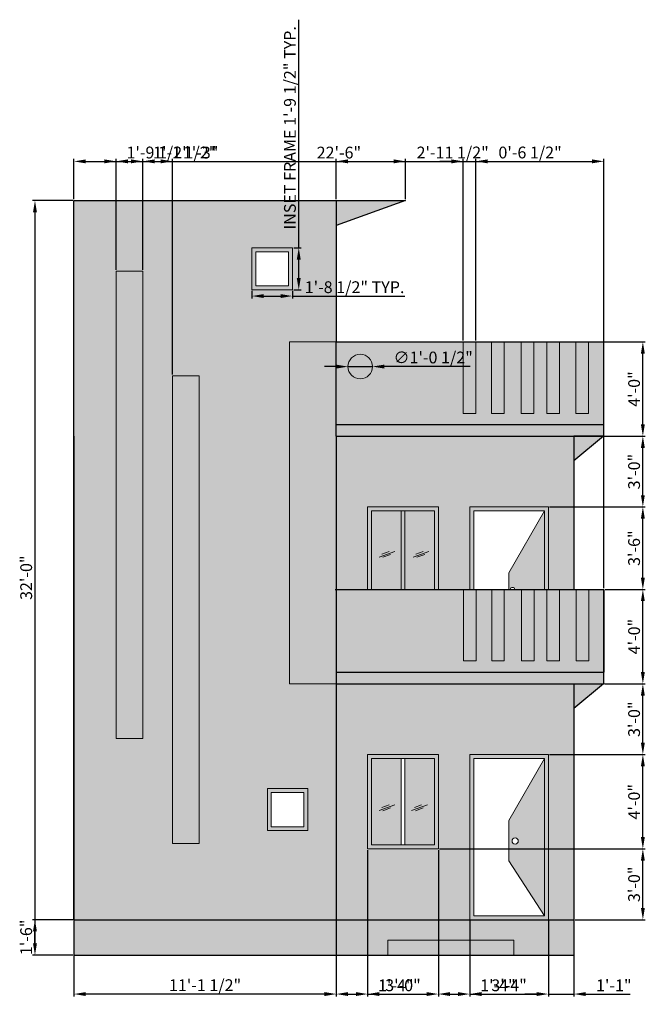
# Model space of a CAD drawing. Units: inches. Extents: x 40559 to 41508, y 131086 to 132358.
# Tile 5 of 5: x 40592 to 40910, y 131857 to 132358. Entities that reach past the tile are written whole.
import ezdxf

# ---------------------------------------------------------------- set-up
doc = ezdxf.new("R2010")
doc.units = ezdxf.units.IN
for name, color, linetype, lineweight in [('A-ANNO-DIMS', 2, 'Continuous', 18), ('A-ELEV', 7, 'Continuous', 30), ('A-ELEV-DETL', 7, 'Continuous', 18), ('A-ELEV-DOOR-PATT', 24, 'Continuous', 13), ('A-ELEV-FRAM-PATT', 7, 'Continuous', 13), ('A-ELEV-OPEN', 7, 'Continuous', 18), ('A-ELEV-RECS-PATT', 250, 'Continuous', 13)]:
    doc.layers.add(name, color=color, linetype=linetype, lineweight=lineweight)
for name, color, linetype, lineweight, true_color in [('A-ELEV-CLAD-PATT', 251, 'Continuous', 13, 0x636466), ('A-ELEV-GLAZ-PATT', 141, 'Continuous', 13, 0xadddf7), ('A-ELEV-TRIM-PATT', 244, 'Continuous', 13, 0x991b1e), ('A-ELEV-WALL-PATT', 254, 'Continuous', 13, 0xfeeab9)]:
    doc.layers.add(name, color=color, linetype=linetype, lineweight=lineweight, true_color=true_color)
doc.styles.get("Standard").update_dxf_attribs({"font": 'arial.ttf'})
doc.dimstyles.new('ISO-25', dxfattribs={"dimtxt": 6, "dimasz": 6, "dimexe": 1.25, "dimexo": 0.625, "dimtad": 1, "dimdec": 0, "dimlunit": 3, "dimtxsty": 'Standard', "dimcen": 2.5, "dimclrd": 1, "dimclre": 1, "dimclrt": 2, "dimadec": 0, "dimazin": 0, "dimtfac": 1, "dimtdec": 0, "dimtmove": 0, "dimatfit": 3, "dimfxl": 1, "dimarcsym": 0})

# ---------------------------------------------------------------- blocks, each defined once
blk = doc.blocks.new('GLAZING-REFLECTION')
for p, q in [((0, 0.1), (8.04, 3.02)), ((1.38, 1.64), (5.11, 3)), ((1.93, 0), (5.91, 1.45))]:
    blk.add_line(p, q)
blk = doc.blocks.new('FACADE-INSET-FRAME')
for points in [[(0, 21.37), (20.63, 21.37), (20.63, 0), (0, 0)], [(2, 19.37), (18.63, 19.37), (18.63, 2), (2, 2)]]:
    blk.add_lwpolyline(points, close=True)
blk = doc.blocks.new('*D62')
at = {"layer": 'A-ANNO-DIMS', "color": 1, "lineweight": -2, "transparency": 16777216}
for p, q in [((40733.88, 132242.44), (40733.88, 132358.49)), ((40731.3, 132242.44), (40735.13, 132242.44)), ((40733.88, 132227.08), (40733.88, 132236.44)), ((40731.3, 132221.08), (40735.13, 132221.08))]:
    blk.add_line(p, q, dxfattribs=at)
at = {"layer": 'A-ANNO-DIMS', "color": 1, "transparency": 16777216}
for points in [[(40732.88, 132236.44), (40734.88, 132236.44), (40733.88, 132242.44)], [(40732.88, 132227.08), (40734.88, 132227.08), (40733.88, 132221.08)]]:
    blk.add_solid(points, dxfattribs=at)
at = {"layer": 'Defpoints', "color": 0, "transparency": 16777216}
for p in [(40730.68, 132242.44), (40733.88, 132242.44), (40730.68, 132221.08)]:
    blk.add_point(p, dxfattribs=at)
at = {"layer": 'A-ANNO-DIMS', "color": 2, "transparency": 16777216, "insert": (40730.16, 132303.47), "char_height": 6, "attachment_point": 5, "rotation": 90}
blk.add_mtext('INSET FRAME 1\'-9 1/2" TYP.', dxfattribs=at)
blk = doc.blocks.new('*D63')
at = {"layer": 'A-ANNO-DIMS', "color": 1, "lineweight": -2, "transparency": 16777216}
for p, q in [((40710.05, 132220.45), (40710.05, 132216.62)), ((40716.05, 132217.87), (40724.68, 132217.87)), ((40730.68, 132220.45), (40730.68, 132216.62)), ((40730.68, 132217.87), (40787.92, 132217.87))]:
    blk.add_line(p, q, dxfattribs=at)
at = {"layer": 'A-ANNO-DIMS', "color": 1, "transparency": 16777216}
for points in [[(40716.05, 132218.87), (40716.05, 132216.87), (40710.05, 132217.87)], [(40724.68, 132218.87), (40724.68, 132216.87), (40730.68, 132217.87)]]:
    blk.add_solid(points, dxfattribs=at)
at = {"layer": 'Defpoints', "color": 0, "transparency": 16777216}
for p in [(40710.05, 132221.08), (40730.68, 132221.08), (40730.68, 132217.87)]:
    blk.add_point(p, dxfattribs=at)
at = {"layer": 'A-ANNO-DIMS', "color": 2, "transparency": 16777216, "insert": (40762.3, 132221.6), "char_height": 6, "attachment_point": 5}
blk.add_mtext('1\'-8 1/2" TYP.', dxfattribs=at)
blk = doc.blocks.new('*D82')
at = {"layer": 'A-ANNO-DIMS', "color": 1, "lineweight": -2, "transparency": 16777216}
for p, q in [((40618.81, 132266.55), (40598.34, 132266.55)), ((40599.59, 132260.55), (40599.59, 131888.55)), ((40618.81, 131882.55), (40598.34, 131882.55))]:
    blk.add_line(p, q, dxfattribs=at)
at = {"layer": 'A-ANNO-DIMS', "color": 1, "transparency": 16777216}
for points in [[(40598.59, 132260.55), (40600.59, 132260.55), (40599.59, 132266.55)], [(40598.59, 131888.55), (40600.59, 131888.55), (40599.59, 131882.55)]]:
    blk.add_solid(points, dxfattribs=at)
at = {"layer": 'Defpoints', "color": 0, "transparency": 16777216}
for p in [(40619.44, 132266.55), (40599.59, 131882.55), (40619.44, 131882.55)]:
    blk.add_point(p, dxfattribs=at)
at = {"layer": 'A-ANNO-DIMS', "color": 2, "transparency": 16777216, "insert": (40595.9, 132074.55), "char_height": 6, "attachment_point": 5, "rotation": 90}
blk.add_mtext('32\'-0"', dxfattribs=at)
blk = doc.blocks.new('*D83')
at = {"layer": 'A-ANNO-DIMS', "color": 1, "lineweight": -2, "transparency": 16777216}
for p, q in [((40619.44, 132267.18), (40619.44, 132287.65)), ((40889.21, 132069.25), (40889.21, 132287.65)), ((40625.44, 132286.4), (40883.21, 132286.4))]:
    blk.add_line(p, q, dxfattribs=at)
at = {"layer": 'A-ANNO-DIMS', "color": 1, "transparency": 16777216}
for points in [[(40625.44, 132287.4), (40625.44, 132285.4), (40619.44, 132286.4)], [(40883.21, 132287.4), (40883.21, 132285.4), (40889.21, 132286.4)]]:
    blk.add_solid(points, dxfattribs=at)
at = {"layer": 'Defpoints', "color": 0, "transparency": 16777216}
for p in [(40889.21, 132286.4), (40619.44, 132266.55), (40889.21, 132068.62)]:
    blk.add_point(p, dxfattribs=at)
at = {"layer": 'A-ANNO-DIMS', "color": 2, "transparency": 16777216, "insert": (40754.32, 132290.09), "char_height": 6, "attachment_point": 5}
blk.add_mtext('22\'-6"', dxfattribs=at)
blk = doc.blocks.new('*D84')
at = {"layer": 'A-ANNO-DIMS', "color": 1, "lineweight": -2, "transparency": 16777216}
for p, q in [((40618.81, 131900.55), (40598.34, 131900.55)), ((40599.59, 131888.55), (40599.59, 131894.55)), ((40618.81, 131882.55), (40598.34, 131882.55))]:
    blk.add_line(p, q, dxfattribs=at)
at = {"layer": 'A-ANNO-DIMS', "color": 1, "transparency": 16777216}
for points in [[(40598.59, 131894.55), (40600.59, 131894.55), (40599.59, 131900.55)], [(40598.59, 131888.55), (40600.59, 131888.55), (40599.59, 131882.55)]]:
    blk.add_solid(points, dxfattribs=at)
at = {"layer": 'Defpoints', "color": 0, "transparency": 16777216}
for p in [(40599.59, 131900.55), (40619.44, 131900.55), (40619.44, 131882.55)]:
    blk.add_point(p, dxfattribs=at)
at = {"layer": 'A-ANNO-DIMS', "color": 2, "transparency": 16777216, "insert": (40595.9, 131891.55), "char_height": 6, "attachment_point": 5, "rotation": 90}
blk.add_mtext('1\'-6"', dxfattribs=at)
blk = doc.blocks.new('*D85')
at = {"layer": 'A-ANNO-DIMS', "color": 1, "lineweight": -2, "transparency": 16777216}
for p, q in [((40889.56, 132020.55), (40910.31, 132020.55)), ((40909.06, 131990.55), (40909.06, 132014.55)), ((40861.56, 131984.55), (40910.31, 131984.55))]:
    blk.add_line(p, q, dxfattribs=at)
at = {"layer": 'A-ANNO-DIMS', "color": 1, "transparency": 16777216}
for points in [[(40908.06, 132014.55), (40910.06, 132014.55), (40909.06, 132020.55)], [(40908.06, 131990.55), (40910.06, 131990.55), (40909.06, 131984.55)]]:
    blk.add_solid(points, dxfattribs=at)
at = {"layer": 'Defpoints', "color": 0, "transparency": 16777216}
for p in [(40888.94, 132020.55), (40909.06, 132020.55), (40860.94, 131984.55)]:
    blk.add_point(p, dxfattribs=at)
at = {"layer": 'A-ANNO-DIMS', "color": 2, "transparency": 16777216, "insert": (40905.37, 132002.55), "char_height": 6, "attachment_point": 5, "rotation": 90}
blk.add_mtext('3\'-0"', dxfattribs=at)
blk = doc.blocks.new('*D86')
at = {"layer": 'A-ANNO-DIMS', "color": 1, "lineweight": -2, "transparency": 16777216}
for p, q in [((40889.83, 132068.62), (40910.31, 132068.62)), ((40909.06, 132026.55), (40909.06, 132062.62)), ((40889.56, 132020.55), (40910.31, 132020.55))]:
    blk.add_line(p, q, dxfattribs=at)
at = {"layer": 'A-ANNO-DIMS', "color": 1, "transparency": 16777216}
for points in [[(40908.06, 132062.62), (40910.06, 132062.62), (40909.06, 132068.62)], [(40908.06, 132026.55), (40910.06, 132026.55), (40909.06, 132020.55)]]:
    blk.add_solid(points, dxfattribs=at)
at = {"layer": 'Defpoints', "color": 0, "transparency": 16777216}
for p in [(40889.21, 132068.62), (40909.06, 132068.62), (40888.94, 132020.55)]:
    blk.add_point(p, dxfattribs=at)
at = {"layer": 'A-ANNO-DIMS', "color": 2, "transparency": 16777216, "insert": (40905.37, 132044.59), "char_height": 6, "attachment_point": 5, "rotation": 90}
blk.add_mtext('4\'-0"', dxfattribs=at)
blk = doc.blocks.new('*D87')
at = {"layer": 'A-ANNO-DIMS', "color": 1, "lineweight": -2, "transparency": 16777216}
for p, q in [((40861.56, 132110.55), (40910.31, 132110.55)), ((40909.06, 132074.62), (40909.06, 132104.55)), ((40889.83, 132068.62), (40910.31, 132068.62))]:
    blk.add_line(p, q, dxfattribs=at)
at = {"layer": 'A-ANNO-DIMS', "color": 1, "transparency": 16777216}
for points in [[(40908.06, 132104.55), (40910.06, 132104.55), (40909.06, 132110.55)], [(40908.06, 132074.62), (40910.06, 132074.62), (40909.06, 132068.62)]]:
    blk.add_solid(points, dxfattribs=at)
at = {"layer": 'Defpoints', "color": 0, "transparency": 16777216}
for p in [(40860.94, 132110.55), (40909.06, 132110.55), (40889.21, 132068.62)]:
    blk.add_point(p, dxfattribs=at)
at = {"layer": 'A-ANNO-DIMS', "color": 2, "transparency": 16777216, "insert": (40905.37, 132089.59), "char_height": 6, "attachment_point": 5, "rotation": 90}
blk.add_mtext('3\'-6"', dxfattribs=at)
blk = doc.blocks.new('*D88')
at = {"layer": 'A-ANNO-DIMS', "color": 1, "lineweight": -2, "transparency": 16777216}
for p, q in [((40889.56, 132146.55), (40910.31, 132146.55)), ((40909.06, 132116.55), (40909.06, 132140.55)), ((40861.56, 132110.55), (40910.31, 132110.55))]:
    blk.add_line(p, q, dxfattribs=at)
at = {"layer": 'A-ANNO-DIMS', "color": 1, "transparency": 16777216}
for points in [[(40908.06, 132140.55), (40910.06, 132140.55), (40909.06, 132146.55)], [(40908.06, 132116.55), (40910.06, 132116.55), (40909.06, 132110.55)]]:
    blk.add_solid(points, dxfattribs=at)
at = {"layer": 'Defpoints', "color": 0, "transparency": 16777216}
for p in [(40888.94, 132146.55), (40909.06, 132146.55), (40860.94, 132110.55)]:
    blk.add_point(p, dxfattribs=at)
at = {"layer": 'A-ANNO-DIMS', "color": 2, "transparency": 16777216, "insert": (40905.37, 132128.55), "char_height": 6, "attachment_point": 5, "rotation": 90}
blk.add_mtext('3\'-0"', dxfattribs=at)
blk = doc.blocks.new('*D89')
at = {"layer": 'A-ANNO-DIMS', "color": 1, "lineweight": -2, "transparency": 16777216}
for p, q in [((40889.56, 132194.55), (40910.31, 132194.55)), ((40909.06, 132152.55), (40909.06, 132188.55)), ((40889.56, 132146.55), (40910.31, 132146.55))]:
    blk.add_line(p, q, dxfattribs=at)
at = {"layer": 'A-ANNO-DIMS', "color": 1, "transparency": 16777216}
for points in [[(40908.06, 132188.55), (40910.06, 132188.55), (40909.06, 132194.55)], [(40908.06, 132152.55), (40910.06, 132152.55), (40909.06, 132146.55)]]:
    blk.add_solid(points, dxfattribs=at)
at = {"layer": 'Defpoints', "color": 0, "transparency": 16777216}
for p in [(40888.94, 132194.55), (40909.06, 132194.55), (40888.94, 132146.55)]:
    blk.add_point(p, dxfattribs=at)
at = {"layer": 'A-ANNO-DIMS', "color": 2, "transparency": 16777216, "insert": (40905.37, 132170.55), "char_height": 6, "attachment_point": 5, "rotation": 90}
blk.add_mtext('4\'-0"', dxfattribs=at)
blk = doc.blocks.new('*D90')
at = {"layer": 'A-ANNO-DIMS', "color": 1, "lineweight": -2, "transparency": 16777216}
for p, q in [((40619.44, 131899.93), (40619.44, 131861.45)), ((40752.94, 131899.93), (40752.94, 131861.45)), ((40746.94, 131862.7), (40625.44, 131862.7))]:
    blk.add_line(p, q, dxfattribs=at)
at = {"layer": 'A-ANNO-DIMS', "color": 1, "transparency": 16777216}
for points in [[(40625.44, 131863.7), (40625.44, 131861.7), (40619.44, 131862.7)], [(40746.94, 131863.7), (40746.94, 131861.7), (40752.94, 131862.7)]]:
    blk.add_solid(points, dxfattribs=at)
at = {"layer": 'Defpoints', "color": 0, "transparency": 16777216}
for p in [(40619.44, 131900.55), (40752.94, 131900.55), (40619.44, 131862.7)]:
    blk.add_point(p, dxfattribs=at)
at = {"layer": 'A-ANNO-DIMS', "color": 2, "transparency": 16777216, "insert": (40686.19, 131866.43), "char_height": 6, "attachment_point": 5}
blk.add_mtext('11\'-1 1/2"', dxfattribs=at)
blk = doc.blocks.new('*D91')
at = {"layer": 'A-ANNO-DIMS', "color": 1, "lineweight": -2, "transparency": 16777216}
for p, q in [((40768.94, 131935.93), (40768.94, 131861.45)), ((40752.94, 131899.93), (40752.94, 131861.45)), ((40758.94, 131862.7), (40762.94, 131862.7)), ((40768.94, 131862.7), (40791.57, 131862.7))]:
    blk.add_line(p, q, dxfattribs=at)
at = {"layer": 'A-ANNO-DIMS', "color": 1, "transparency": 16777216}
for points in [[(40758.94, 131863.7), (40758.94, 131861.7), (40752.94, 131862.7)], [(40762.94, 131863.7), (40762.94, 131861.7), (40768.94, 131862.7)]]:
    blk.add_solid(points, dxfattribs=at)
at = {"layer": 'Defpoints', "color": 0, "transparency": 16777216}
for p in [(40768.94, 131936.55), (40752.94, 131900.55), (40768.94, 131862.7)]:
    blk.add_point(p, dxfattribs=at)
at = {"layer": 'A-ANNO-DIMS', "color": 2, "transparency": 16777216, "insert": (40783.26, 131866.34), "char_height": 6, "attachment_point": 5}
blk.add_mtext('1\'-4"', dxfattribs=at)
blk = doc.blocks.new('*D92')
at = {"layer": 'A-ANNO-DIMS', "color": 1, "lineweight": -2, "transparency": 16777216}
for p, q in [((40768.94, 131935.93), (40768.94, 131861.45)), ((40804.94, 131935.93), (40804.94, 131861.45)), ((40774.94, 131862.7), (40798.94, 131862.7))]:
    blk.add_line(p, q, dxfattribs=at)
at = {"layer": 'A-ANNO-DIMS', "color": 1, "transparency": 16777216}
for points in [[(40774.94, 131863.7), (40774.94, 131861.7), (40768.94, 131862.7)], [(40798.94, 131863.7), (40798.94, 131861.7), (40804.94, 131862.7)]]:
    blk.add_solid(points, dxfattribs=at)
at = {"layer": 'Defpoints', "color": 0, "transparency": 16777216}
for p in [(40768.94, 131936.55), (40804.94, 131936.55), (40804.94, 131862.7)]:
    blk.add_point(p, dxfattribs=at)
at = {"layer": 'A-ANNO-DIMS', "color": 2, "transparency": 16777216, "insert": (40786.94, 131866.39), "char_height": 6, "attachment_point": 5}
blk.add_mtext('3\'-0"', dxfattribs=at)
blk = doc.blocks.new('*D93')
at = {"layer": 'A-ANNO-DIMS', "color": 1, "lineweight": -2, "transparency": 16777216}
for p, q in [((40804.94, 131935.93), (40804.94, 131861.45)), ((40820.94, 131899.93), (40820.94, 131861.45)), ((40810.94, 131862.7), (40814.94, 131862.7)), ((40820.94, 131862.7), (40843.57, 131862.7))]:
    blk.add_line(p, q, dxfattribs=at)
at = {"layer": 'A-ANNO-DIMS', "color": 1, "transparency": 16777216}
for points in [[(40810.94, 131863.7), (40810.94, 131861.7), (40804.94, 131862.7)], [(40814.94, 131863.7), (40814.94, 131861.7), (40820.94, 131862.7)]]:
    blk.add_solid(points, dxfattribs=at)
at = {"layer": 'Defpoints', "color": 0, "transparency": 16777216}
for p in [(40804.94, 131936.55), (40820.94, 131900.55), (40820.94, 131862.7)]:
    blk.add_point(p, dxfattribs=at)
at = {"layer": 'A-ANNO-DIMS', "color": 2, "transparency": 16777216, "insert": (40835.26, 131866.34), "char_height": 6, "attachment_point": 5}
blk.add_mtext('1\'-4"', dxfattribs=at)
blk = doc.blocks.new('*D94')
at = {"layer": 'A-ANNO-DIMS', "color": 1, "lineweight": -2, "transparency": 16777216}
for p, q in [((40820.94, 131899.93), (40820.94, 131861.45)), ((40860.94, 131899.93), (40860.94, 131861.45)), ((40826.94, 131862.7), (40854.94, 131862.7))]:
    blk.add_line(p, q, dxfattribs=at)
at = {"layer": 'A-ANNO-DIMS', "color": 1, "transparency": 16777216}
for points in [[(40826.94, 131863.7), (40826.94, 131861.7), (40820.94, 131862.7)], [(40854.94, 131863.7), (40854.94, 131861.7), (40860.94, 131862.7)]]:
    blk.add_solid(points, dxfattribs=at)
at = {"layer": 'Defpoints', "color": 0, "transparency": 16777216}
for p in [(40820.94, 131900.55), (40860.94, 131900.55), (40860.94, 131862.7)]:
    blk.add_point(p, dxfattribs=at)
at = {"layer": 'A-ANNO-DIMS', "color": 2, "transparency": 16777216, "insert": (40840.94, 131866.39), "char_height": 6, "attachment_point": 5}
blk.add_mtext('3\'-4"', dxfattribs=at)
blk = doc.blocks.new('*D95')
at = {"layer": 'A-ANNO-DIMS', "color": 1, "lineweight": -2, "transparency": 16777216}
for p, q in [((40860.94, 131899.93), (40860.94, 131861.45)), ((40873.94, 131899.93), (40873.94, 131861.45)), ((40854.94, 131862.7), (40848.94, 131862.7)), ((40860.94, 131862.7), (40873.94, 131862.7)), ((40879.94, 131862.7), (40902.57, 131862.7))]:
    blk.add_line(p, q, dxfattribs=at)
at = {"layer": 'A-ANNO-DIMS', "color": 1, "transparency": 16777216}
for points in [[(40854.94, 131863.7), (40854.94, 131861.7), (40860.94, 131862.7)], [(40879.94, 131863.7), (40879.94, 131861.7), (40873.94, 131862.7)]]:
    blk.add_solid(points, dxfattribs=at)
at = {"layer": 'Defpoints', "color": 0, "transparency": 16777216}
for p in [(40860.94, 131900.55), (40873.94, 131900.55), (40873.94, 131862.7)]:
    blk.add_point(p, dxfattribs=at)
at = {"layer": 'A-ANNO-DIMS', "color": 2, "transparency": 16777216, "insert": (40894.26, 131866.34), "char_height": 6, "attachment_point": 5}
blk.add_mtext('1\'-1"', dxfattribs=at)
blk = doc.blocks.new('*D96')
at = {"layer": 'A-ANNO-DIMS', "color": 1, "lineweight": -2, "transparency": 16777216}
for p, q in [((40805.56, 131936.55), (40910.31, 131936.55)), ((40909.06, 131906.55), (40909.06, 131930.55)), ((40874.56, 131900.55), (40910.31, 131900.55))]:
    blk.add_line(p, q, dxfattribs=at)
at = {"layer": 'A-ANNO-DIMS', "color": 1, "transparency": 16777216}
for points in [[(40908.06, 131930.55), (40910.06, 131930.55), (40909.06, 131936.55)], [(40908.06, 131906.55), (40910.06, 131906.55), (40909.06, 131900.55)]]:
    blk.add_solid(points, dxfattribs=at)
at = {"layer": 'Defpoints', "color": 0, "transparency": 16777216}
for p in [(40804.94, 131936.55), (40909.06, 131936.55), (40873.94, 131900.55)]:
    blk.add_point(p, dxfattribs=at)
at = {"layer": 'A-ANNO-DIMS', "color": 2, "transparency": 16777216, "insert": (40905.37, 131918.55), "char_height": 6, "attachment_point": 5, "rotation": 90}
blk.add_mtext('3\'-0"', dxfattribs=at)
blk = doc.blocks.new('*D97')
at = {"layer": 'A-ANNO-DIMS', "color": 1, "lineweight": -2, "transparency": 16777216}
for p, q in [((40861.56, 131984.55), (40910.31, 131984.55)), ((40909.06, 131942.55), (40909.06, 131978.55)), ((40805.56, 131936.55), (40910.31, 131936.55))]:
    blk.add_line(p, q, dxfattribs=at)
at = {"layer": 'A-ANNO-DIMS', "color": 1, "transparency": 16777216}
for points in [[(40908.06, 131978.55), (40910.06, 131978.55), (40909.06, 131984.55)], [(40908.06, 131942.55), (40910.06, 131942.55), (40909.06, 131936.55)]]:
    blk.add_solid(points, dxfattribs=at)
at = {"layer": 'Defpoints', "color": 0, "transparency": 16777216}
for p in [(40860.94, 131984.55), (40909.06, 131984.55), (40804.94, 131936.55)]:
    blk.add_point(p, dxfattribs=at)
at = {"layer": 'A-ANNO-DIMS', "color": 2, "transparency": 16777216, "insert": (40905.37, 131960.55), "char_height": 6, "attachment_point": 5, "rotation": 90}
blk.add_mtext('4\'-0"', dxfattribs=at)
blk = doc.blocks.new('*D98')
at = {"layer": 'A-ANNO-DIMS', "color": 1, "lineweight": -2, "transparency": 16777216}
for p, q in [((40817.63, 132195.18), (40817.63, 132287.65)), ((40824.05, 132195.18), (40824.05, 132287.65)), ((40811.63, 132286.4), (40805.63, 132286.4)), ((40817.63, 132286.4), (40824.05, 132286.4)), ((40830.05, 132286.4), (40867.23, 132286.4))]:
    blk.add_line(p, q, dxfattribs=at)
at = {"layer": 'A-ANNO-DIMS', "color": 1, "transparency": 16777216}
for points in [[(40811.63, 132287.4), (40811.63, 132285.4), (40817.63, 132286.4)], [(40830.05, 132287.4), (40830.05, 132285.4), (40824.05, 132286.4)]]:
    blk.add_solid(points, dxfattribs=at)
at = {"layer": 'Defpoints', "color": 0, "transparency": 16777216}
for p in [(40824.05, 132286.4), (40817.63, 132194.55), (40824.05, 132194.55)]:
    blk.add_point(p, dxfattribs=at)
at = {"layer": 'A-ANNO-DIMS', "color": 2, "transparency": 16777216, "insert": (40851.64, 132290.13), "char_height": 6, "attachment_point": 5}
blk.add_mtext('0\'-6 1/2"', dxfattribs=at)
blk = doc.blocks.new('*D99')
at = {"layer": 'A-ANNO-DIMS', "color": 1, "lineweight": -2, "transparency": 16777216}
for p, q in [((40752.94, 132267.18), (40752.94, 132287.65)), ((40788.26, 132267.18), (40788.26, 132287.65)), ((40758.94, 132286.4), (40782.26, 132286.4)), ((40788.26, 132286.4), (40830.21, 132286.4))]:
    blk.add_line(p, q, dxfattribs=at)
at = {"layer": 'A-ANNO-DIMS', "color": 1, "transparency": 16777216}
for points in [[(40758.94, 132287.4), (40758.94, 132285.4), (40752.94, 132286.4)], [(40782.26, 132287.4), (40782.26, 132285.4), (40788.26, 132286.4)]]:
    blk.add_solid(points, dxfattribs=at)
at = {"layer": 'Defpoints', "color": 0, "transparency": 16777216}
for p in [(40788.26, 132286.4), (40752.94, 132266.55), (40788.26, 132266.55)]:
    blk.add_point(p, dxfattribs=at)
at = {"layer": 'A-ANNO-DIMS', "color": 2, "transparency": 16777216, "insert": (40812.23, 132290.13), "char_height": 6, "attachment_point": 5}
blk.add_mtext('2\'-11 1/2"', dxfattribs=at)
blk = doc.blocks.new('*D100')
at = {"layer": 'A-ANNO-DIMS', "color": 1, "lineweight": -2, "transparency": 16777216}
for p, q in [((40640.97, 132231.22), (40640.97, 132287.65)), ((40654.52, 132231.22), (40654.52, 132287.65)), ((40646.97, 132286.4), (40648.52, 132286.4)), ((40654.52, 132286.4), (40691.13, 132286.4))]:
    blk.add_line(p, q, dxfattribs=at)
at = {"layer": 'A-ANNO-DIMS', "color": 1, "transparency": 16777216}
for points in [[(40646.97, 132287.4), (40646.97, 132285.4), (40640.97, 132286.4)], [(40648.52, 132287.4), (40648.52, 132285.4), (40654.52, 132286.4)]]:
    blk.add_solid(points, dxfattribs=at)
at = {"layer": 'Defpoints', "color": 0, "transparency": 16777216}
for p in [(40654.52, 132286.4), (40640.97, 132230.6), (40654.52, 132230.6)]:
    blk.add_point(p, dxfattribs=at)
at = {"layer": 'A-ANNO-DIMS', "color": 2, "transparency": 16777216, "insert": (40675.82, 132290.13), "char_height": 6, "attachment_point": 5}
blk.add_mtext('1\'-1 1/2"', dxfattribs=at)
blk = doc.blocks.new('*D101')
at = {"layer": 'A-ANNO-DIMS', "color": 1, "lineweight": -2, "transparency": 16777216}
for p, q in [((40619.44, 132267.18), (40619.44, 132287.65)), ((40640.97, 132231.22), (40640.97, 132287.65)), ((40625.44, 132286.4), (40634.97, 132286.4)), ((40640.97, 132286.4), (40677.58, 132286.4))]:
    blk.add_line(p, q, dxfattribs=at)
at = {"layer": 'A-ANNO-DIMS', "color": 1, "transparency": 16777216}
for points in [[(40625.44, 132287.4), (40625.44, 132285.4), (40619.44, 132286.4)], [(40634.97, 132287.4), (40634.97, 132285.4), (40640.97, 132286.4)]]:
    blk.add_solid(points, dxfattribs=at)
at = {"layer": 'Defpoints', "color": 0, "transparency": 16777216}
for p in [(40640.97, 132286.4), (40619.44, 132266.55), (40640.97, 132230.6)]:
    blk.add_point(p, dxfattribs=at)
at = {"layer": 'A-ANNO-DIMS', "color": 2, "transparency": 16777216, "insert": (40662.28, 132290.13), "char_height": 6, "attachment_point": 5}
blk.add_mtext('1\'-9 1/2"', dxfattribs=at)
blk = doc.blocks.new('*D102')
at = {"layer": 'A-ANNO-DIMS', "color": 1, "lineweight": -2, "transparency": 16777216}
for p, q in [((40654.52, 132231.22), (40654.52, 132287.65)), ((40669.6, 132177.9), (40669.6, 132287.65)), ((40660.52, 132286.4), (40663.6, 132286.4)), ((40669.6, 132286.4), (40692.23, 132286.4))]:
    blk.add_line(p, q, dxfattribs=at)
at = {"layer": 'A-ANNO-DIMS', "color": 1, "transparency": 16777216}
for points in [[(40660.52, 132287.4), (40660.52, 132285.4), (40654.52, 132286.4)], [(40663.6, 132287.4), (40663.6, 132285.4), (40669.6, 132286.4)]]:
    blk.add_solid(points, dxfattribs=at)
at = {"layer": 'Defpoints', "color": 0, "transparency": 16777216}
for p in [(40669.6, 132286.4), (40654.52, 132230.6), (40669.6, 132177.27)]:
    blk.add_point(p, dxfattribs=at)
at = {"layer": 'A-ANNO-DIMS', "color": 2, "transparency": 16777216, "insert": (40683.92, 132290.09), "char_height": 6, "attachment_point": 5}
blk.add_mtext('1\'-3"', dxfattribs=at)
blk = doc.blocks.new('*D106')
at = {"layer": 'A-ANNO-DIMS', "color": 1, "lineweight": -2, "transparency": 16777216}
for p, q in [((40752.93, 132181.97), (40746.93, 132181.97)), ((40758.93, 132181.97), (40771.44, 132181.97)), ((40821.15, 132181.97), (40777.44, 132181.97))]:
    blk.add_line(p, q, dxfattribs=at)
at = {"layer": 'A-ANNO-DIMS', "color": 1, "transparency": 16777216}
for points in [[(40752.93, 132182.97), (40752.93, 132180.97), (40758.93, 132181.97)], [(40777.44, 132182.97), (40777.44, 132180.97), (40771.44, 132181.97)]]:
    blk.add_solid(points, dxfattribs=at)
at = {"layer": 'Defpoints', "color": 0, "transparency": 16777216}
for p in [(40758.93, 132181.97), (40771.44, 132181.97)]:
    blk.add_point(p, dxfattribs=at)
at = {"layer": 'A-ANNO-DIMS', "color": 2, "transparency": 16777216, "insert": (40802.3, 132185.83), "char_height": 6, "attachment_point": 5, "rotation": 0.001}
blk.add_mtext('∅1\'-0 1/2"', dxfattribs=at)

msp = doc.modelspace()

# ---------------------------------------------------------------- hatches: boundary and pattern name
at = {"layer": 'A-ELEV-CLAD-PATT'}
h = msp.add_hatch(color=256, dxfattribs=at)
h.dxf.hatch_style = 1
h.paths.add_polyline_path([(40729.2, 132194.55), (40752.94, 132194.55), (40752.94, 132266.55), (40619.44, 132266.55), (40619.44, 132194.55), (40619.44, 132146.55), (40619.44, 132020.55), (40619.44, 131900.55), (40752.94, 131900.55), (40752.94, 132020.55), (40729.2, 132020.55)])
h.paths.add_polyline_path([(40683.15, 132177.27), (40683.15, 131939.36), (40669.6, 131939.36), (40669.6, 132177.27)], flags=16)
h.paths.add_polyline_path([(40710.05, 132221.08), (40710.05, 132242.44), (40730.68, 132242.44), (40730.68, 132221.08)], flags=16)
h.paths.add_polyline_path([(40712.05, 132223.08), (40712.05, 132240.44), (40728.68, 132240.44), (40728.68, 132223.08)], flags=0)
h.paths.add_polyline_path([(40654.52, 131992.69), (40640.97, 131992.69), (40640.97, 132230.6), (40654.52, 132230.6)], flags=16)
h.paths.add_polyline_path([(40717.89, 131967.22), (40738.52, 131967.22), (40738.52, 131945.85), (40717.89, 131945.85)], flags=16)
h.paths.add_polyline_path([(40719.89, 131965.22), (40736.52, 131965.22), (40736.52, 131947.85), (40719.89, 131947.85)], flags=0)
h = msp.add_hatch(color=256, dxfattribs=at)
h.dxf.hatch_style = 1
h.paths.add_polyline_path([(40817.69, 132068.55), (40752.94, 132068.55), (40752.94, 132026.55), (40888.94, 132026.55), (40888.94, 132068.55), (40881.5, 132068.55), (40881.5, 132032.18), (40875.08, 132032.18), (40875.08, 132068.55), (40873.94, 132068.55), (40866.62, 132068.55), (40866.62, 132032.18), (40860.2, 132032.18), (40860.2, 132068.55), (40853.65, 132068.55), (40853.65, 132032.18), (40847.23, 132032.18), (40847.23, 132068.55), (40838.53, 132068.55), (40838.53, 132032.18), (40832.1, 132032.18), (40832.1, 132068.55), (40824.12, 132068.55), (40824.12, 132032.18), (40817.69, 132032.18)])
h.paths.add_polyline_path([(40817.63, 132194.55), (40752.94, 132194.55), (40752.94, 132152.55), (40888.94, 132152.55), (40888.94, 132194.55), (40881.44, 132194.55), (40881.44, 132158.11), (40875.01, 132158.11), (40875.01, 132194.55), (40866.56, 132194.55), (40866.56, 132158.11), (40860.13, 132158.11), (40860.13, 132194.55), (40853.59, 132194.55), (40853.59, 132158.11), (40847.16, 132158.11), (40847.16, 132194.55), (40838.46, 132194.55), (40838.46, 132158.11), (40832.03, 132158.11), (40832.03, 132194.55), (40824.05, 132194.55), (40824.05, 132158.11), (40817.63, 132158.11)])
h.paths.add_polyline_path([(40758.93, 132181.97, -1), (40771.44, 132181.97, -1)], flags=16)
h = msp.add_hatch(color=256, dxfattribs=at)
h.dxf.hatch_style = 1
h.paths.add_polyline_path([(40873.94, 131900.55), (40619.44, 131900.55), (40619.44, 131882.55), (40779.29, 131882.55), (40779.29, 131890.06), (40843.37, 131890.06), (40843.37, 131882.55), (40873.94, 131882.55)])
at = {"layer": 'A-ELEV-DOOR-PATT'}
h = msp.add_hatch(color=256, dxfattribs=at)
h.dxf.hatch_style = 1
h.paths.add_polyline_path([(40858.94, 131982.55), (40840.76, 131951.07), (40840.76, 131930.45), (40858.94, 131902.55)])
h.paths.add_polyline_path([(40845.62, 131940.52, -1), (40842.44, 131940.52, -1)], flags=16)
h.paths.add_polyline_path([(40858.94, 132108.55), (40840.76, 132077.07), (40840.76, 132068.55), (40841.6, 132068.55, -1), (40843.79, 132068.55), (40858.94, 132068.55)])
at = {"layer": 'A-ELEV-FRAM-PATT'}
h = msp.add_hatch(color=256, dxfattribs=at)
h.dxf.hatch_style = 1
h.paths.add_polyline_path([(40804.94, 132110.55), (40768.94, 132110.55), (40768.94, 132068.55), (40770.94, 132068.55), (40770.94, 132108.55), (40802.94, 132108.55), (40802.94, 132068.55), (40804.94, 132068.55)])
h.paths.add_polyline_path([(40787.94, 132108.55), (40785.94, 132108.55), (40785.94, 132068.55), (40787.94, 132068.55)], flags=17)
h.paths.add_polyline_path([(40804.94, 131984.55), (40768.94, 131984.55), (40768.94, 131936.55), (40804.94, 131936.55)])
h.paths.add_polyline_path([(40802.94, 131982.55), (40802.94, 131938.55), (40770.94, 131938.55), (40770.94, 131982.55)], flags=16)
h.paths.add_polyline_path([(40787.94, 131982.55), (40785.94, 131982.55), (40785.94, 131938.55), (40787.94, 131938.55)], flags=0)
h = msp.add_hatch(color=256, dxfattribs=at)
h.dxf.hatch_style = 1
h.paths.add_polyline_path([(40860.94, 132110.55), (40820.94, 132110.55), (40820.94, 132068.55), (40822.94, 132068.55), (40822.94, 132108.55), (40858.94, 132108.55), (40858.94, 132068.55), (40860.94, 132068.55)])
h.paths.add_polyline_path([(40860.94, 131984.55), (40820.94, 131984.55), (40820.94, 131900.55), (40860.94, 131900.55)])
h.paths.add_polyline_path([(40858.94, 131982.55), (40858.94, 131902.55), (40822.94, 131902.55), (40822.94, 131982.55)], flags=16)
h.paths.add_polyline_path([(40845.62, 131940.52, -1), (40842.44, 131940.52, -1)], flags=0)
at = {"layer": 'A-ELEV-GLAZ-PATT'}
h = msp.add_hatch(color=256, dxfattribs=at)
h.dxf.hatch_style = 1
h.paths.add_polyline_path([(40785.94, 132108.55), (40770.94, 132108.55), (40770.94, 132068.55), (40785.94, 132068.55)])
h.paths.add_polyline_path([(40802.94, 132108.55), (40787.94, 132108.55), (40787.94, 132068.55), (40802.94, 132068.55)])
h.paths.add_polyline_path([(40785.94, 131982.55), (40770.94, 131982.55), (40770.94, 131938.55), (40785.94, 131938.55)])
h.paths.add_polyline_path([(40802.94, 131982.55), (40787.94, 131982.55), (40787.94, 131938.55), (40802.94, 131938.55)])
at = {"layer": 'A-ELEV-RECS-PATT'}
h = msp.add_hatch(color=256, dxfattribs=at)
h.dxf.hatch_style = 1
h.paths.add_polyline_path([(40788.26, 132266.55), (40777.38, 132266.55), (40752.94, 132266.55), (40752.94, 132253.7)])
h = msp.add_hatch(color=256, dxfattribs=at)
h.dxf.hatch_style = 1
h.paths.add_polyline_path([(40654.52, 132230.6), (40640.97, 132230.6), (40640.97, 131992.69), (40654.52, 131992.69)])
h = msp.add_hatch(color=256, dxfattribs=at)
h.dxf.hatch_style = 1
h.paths.add_polyline_path([(40683.15, 132177.27), (40669.6, 132177.27), (40669.6, 131939.36), (40683.15, 131939.36)])
h = msp.add_hatch(color=256, dxfattribs=at)
h.dxf.hatch_style = 1
h.paths.add_polyline_path([(40888.94, 132146.55), (40873.94, 132146.55), (40873.94, 132133.97)])
h.paths.add_polyline_path([(40888.94, 132020.55), (40873.94, 132020.55), (40873.94, 132007.97)])
h = msp.add_hatch(color=256, dxfattribs=at)
h.dxf.hatch_style = 1
h.paths.add_polyline_path([(40843.37, 131890.06), (40779.29, 131890.06), (40779.29, 131882.55), (40843.37, 131882.55)])
at = {"layer": 'A-ELEV-TRIM-PATT'}
h = msp.add_hatch(color=256, dxfattribs=at)
h.dxf.hatch_style = 1
h.paths.add_polyline_path([(40738.52, 131967.22), (40717.89, 131967.22), (40717.89, 131945.85), (40738.52, 131945.85)])
h.paths.add_polyline_path([(40736.52, 131965.22), (40736.52, 131947.85), (40719.89, 131947.85), (40719.89, 131965.22)], flags=16)
h.paths.add_polyline_path([(40730.68, 132242.44), (40710.05, 132242.44), (40710.05, 132221.08), (40730.68, 132221.08)])
h.paths.add_polyline_path([(40728.68, 132240.44), (40728.68, 132223.08), (40712.05, 132223.08), (40712.05, 132240.44)], flags=16)
h = msp.add_hatch(color=256, dxfattribs=at)
h.dxf.hatch_style = 1
h.paths.add_polyline_path([(40752.94, 132146.55), (40752.94, 132194.55), (40729.2, 132194.55), (40729.2, 132020.55), (40752.94, 132020.55)])
h = msp.add_hatch(color=256, dxfattribs=at)
h.dxf.hatch_style = 1
h.paths.add_polyline_path([(40824.05, 132194.55), (40817.63, 132194.55), (40817.63, 132158.11), (40824.05, 132158.11)])
h.paths.add_polyline_path([(40838.46, 132194.55), (40832.03, 132194.55), (40832.03, 132158.11), (40838.46, 132158.11)])
h.paths.add_polyline_path([(40853.59, 132194.55), (40847.16, 132194.55), (40847.16, 132158.11), (40853.59, 132158.11)])
h.paths.add_polyline_path([(40866.56, 132194.55), (40860.13, 132194.55), (40860.13, 132158.11), (40866.56, 132158.11)])
h.paths.add_polyline_path([(40881.44, 132194.55), (40875.01, 132194.55), (40875.01, 132158.11), (40881.44, 132158.11)])
h.paths.add_polyline_path([(40758.93, 132181.97, 1), (40771.44, 132181.97, 1)])
h = msp.add_hatch(color=256, dxfattribs=at)
h.dxf.hatch_style = 1
h.paths.add_polyline_path([(40888.94, 132026.55), (40752.94, 132026.55), (40752.94, 132020.55), (40888.94, 132020.55)])
h.paths.add_polyline_path([(40888.94, 132152.55), (40752.94, 132152.55), (40752.94, 132146.55), (40888.94, 132146.55)])
h = msp.add_hatch(color=256, dxfattribs=at)
h.dxf.hatch_style = 1
h.paths.add_polyline_path([(40824.12, 132068.55), (40817.69, 132068.55), (40817.69, 132032.18), (40824.12, 132032.18)])
h.paths.add_polyline_path([(40838.53, 132068.55), (40832.1, 132068.55), (40832.1, 132032.18), (40838.53, 132032.18)])
h.paths.add_polyline_path([(40853.65, 132068.55), (40847.23, 132068.55), (40847.23, 132032.18), (40853.65, 132032.18)])
h.paths.add_polyline_path([(40866.62, 132068.55), (40860.2, 132068.55), (40860.2, 132032.18), (40866.62, 132032.18)])
h.paths.add_polyline_path([(40881.5, 132068.55), (40875.08, 132068.55), (40875.08, 132032.18), (40881.5, 132032.18)])
at = {"layer": 'A-ELEV-WALL-PATT'}
h = msp.add_hatch(color=256, dxfattribs=at)
h.dxf.hatch_style = 1
h.paths.add_polyline_path([(40873.94, 132146.55), (40752.94, 132146.55), (40752.94, 132068.55), (40768.94, 132068.55), (40768.94, 132110.55), (40804.94, 132110.55), (40804.94, 132068.55), (40820.94, 132068.55), (40820.94, 132110.55), (40860.94, 132110.55), (40860.94, 132068.55), (40873.94, 132068.55)])
h.paths.add_polyline_path([(40873.94, 132020.55), (40752.94, 132020.55), (40752.94, 131900.55), (40820.94, 131900.55), (40820.94, 131984.55), (40860.94, 131984.55), (40860.94, 131900.55), (40873.94, 131900.55)])
h.paths.add_polyline_path([(40804.94, 131984.55), (40804.94, 131936.55), (40768.94, 131936.55), (40768.94, 131984.55)], flags=16)
h.paths.add_polyline_path([(40802.94, 131982.55), (40802.94, 131938.55), (40770.94, 131938.55), (40770.94, 131982.55)], flags=0)

# ---------------------------------------------------------------- linework, layer by layer
at = {"layer": 'A-ELEV'}
for p, q in [((40619.44, 132194.55), (40619.44, 132266.55)), ((40619.44, 132266.55), (40752.94, 132266.55)), ((40619.44, 131900.55), (40619.44, 132266.55)), ((40619.44, 132266.55), (40788.26, 132266.55)), ((40752.94, 132266.55), (40752.94, 132194.55)), ((40752.94, 132266.55), (40777.38, 132266.55)), ((40788.26, 132266.55), (40752.94, 132253.7)), ((40752.94, 132266.55), (40752.94, 132194.55)), ((40777.38, 132266.55), (40788.26, 132266.55)), ((40619.44, 132146.55), (40619.44, 132194.55)), ((40752.94, 132194.55), (40873.94, 132194.55)), ((40752.94, 132146.55), (40752.94, 132194.55)), ((40752.94, 132194.55), (40888.94, 132194.55)), ((40873.94, 132194.55), (40888.94, 132194.55)), ((40888.94, 132194.55), (40888.94, 132146.55)), ((40888.94, 132194.55), (40888.94, 132152.55)), ((40752.94, 132152.55), (40888.94, 132152.55)), ((40619.44, 132146.55), (40619.44, 132020.55)), ((40752.94, 132146.55), (40752.94, 132020.55)), ((40752.94, 132146.55), (40888.94, 132146.55)), ((40873.94, 132146.55), (40873.94, 132068.55)), ((40888.94, 132146.55), (40873.94, 132146.55)), ((40888.94, 132146.55), (40873.94, 132133.97)), ((40752.37, 132068.62), (40889.21, 132068.62)), ((40752.94, 132068.55), (40889.21, 132068.62)), ((40752.94, 132068.55), (40873.94, 132068.55)), ((40873.94, 132068.55), (40888.94, 132068.55)), ((40888.94, 132068.55), (40888.94, 132020.55)), ((40889.21, 132068.62), (40889.21, 132026.55)), ((40752.94, 132026.55), (40888.94, 132026.55)), ((40752.94, 132026.55), (40888.94, 132026.55)), ((40619.44, 132020.55), (40619.44, 131900.55)), ((40752.94, 132020.55), (40888.94, 132020.55)), ((40752.94, 132020.55), (40752.94, 131900.55)), ((40873.94, 132020.55), (40873.94, 131900.55)), ((40888.94, 132020.55), (40873.94, 132007.97)), ((40873.94, 132007.97), (40873.94, 131900.55)), ((40619.44, 131900.55), (40873.94, 131900.55)), ((40619.44, 131900.55), (40619.44, 131882.55)), ((40619.44, 131900.55), (40873.94, 131900.55)), ((40873.94, 131900.55), (40873.94, 131882.55)), ((40619.44, 131882.55), (40873.94, 131882.55))]:
    msp.add_line(p, q, dxfattribs=at)
at = {"layer": 'A-ELEV-DETL'}
for p, q in [((40640.97, 132230.6), (40654.52, 132230.6)), ((40752.94, 132194.55), (40729.2, 132194.55)), ((40729.2, 132194.55), (40729.2, 132020.55)), ((40752.94, 132194.55), (40729.2, 132194.55)), ((40729.2, 132194.55), (40729.2, 132020.55)), ((40669.6, 132177.27), (40683.15, 132177.27)), ((40729.2, 132020.55), (40752.94, 132020.55)), ((40729.2, 132020.55), (40752.94, 132020.55))]:
    msp.add_line(p, q, dxfattribs=at)
for points in [[(40640.97, 132230.6), (40654.52, 132230.6), (40654.52, 131992.69), (40640.97, 131992.69)], [(40640.97, 132230.6), (40654.52, 132230.6), (40654.52, 131992.69), (40640.97, 131992.69)], [(40640.97, 132230.6), (40654.52, 132230.6), (40654.52, 131992.69), (40640.97, 131992.69)], [(40817.63, 132194.55), (40824.05, 132194.55), (40824.05, 132158.11), (40817.63, 132158.11)], [(40817.63, 132194.55), (40824.05, 132194.55), (40824.05, 132158.11), (40817.63, 132158.11)], [(40832.03, 132194.55), (40838.46, 132194.55), (40838.46, 132158.11), (40832.03, 132158.11)], [(40832.03, 132194.55), (40838.46, 132194.55), (40838.46, 132158.11), (40832.03, 132158.11)], [(40847.16, 132194.55), (40853.59, 132194.55), (40853.59, 132158.11), (40847.16, 132158.11)], [(40847.16, 132194.55), (40853.59, 132194.55), (40853.59, 132158.11), (40847.16, 132158.11)], [(40860.13, 132194.55), (40866.56, 132194.55), (40866.56, 132158.11), (40860.13, 132158.11)], [(40860.13, 132194.55), (40866.56, 132194.55), (40866.56, 132158.11), (40860.13, 132158.11)], [(40875.01, 132194.55), (40881.44, 132194.55), (40881.44, 132158.11), (40875.01, 132158.11)], [(40875.01, 132194.55), (40881.44, 132194.55), (40881.44, 132158.11), (40875.01, 132158.11)], [(40669.6, 132177.27), (40683.15, 132177.27), (40683.15, 131939.36), (40669.6, 131939.36)], [(40669.6, 132177.27), (40683.15, 132177.27), (40683.15, 131939.36), (40669.6, 131939.36)], [(40817.69, 132068.62), (40824.12, 132068.62), (40824.12, 132032.18), (40817.69, 132032.18)], [(40832.1, 132068.62), (40838.53, 132068.62), (40838.53, 132032.18), (40832.1, 132032.18)], [(40847.23, 132068.62), (40853.65, 132068.62), (40853.65, 132032.18), (40847.23, 132032.18)], [(40860.2, 132068.62), (40866.62, 132068.62), (40866.62, 132032.18), (40860.2, 132032.18)], [(40875.08, 132068.62), (40881.5, 132068.62), (40881.5, 132032.18), (40875.08, 132032.18)], [(40779.29, 131882.55), (40843.37, 131882.55), (40843.37, 131890.06), (40779.29, 131890.06)]]:
    msp.add_lwpolyline(points, close=True, dxfattribs=at)
msp.add_circle((40765.19, 132181.97), 6.25, dxfattribs=at)
at = {"layer": 'A-ELEV-OPEN'}
for p, q in [((40768.94, 132068.55), (40768.94, 132110.55)), ((40768.94, 132110.55), (40804.94, 132110.55)), ((40785.94, 132108.55), (40785.94, 132068.55)), ((40787.94, 132108.55), (40787.94, 132068.55)), ((40804.94, 132110.55), (40804.94, 132068.55)), ((40820.94, 132068.55), (40820.94, 132110.55)), ((40820.94, 132110.55), (40860.94, 132110.55)), ((40860.94, 132110.55), (40860.94, 132068.55)), ((40768.94, 131936.55), (40768.94, 131984.55)), ((40768.94, 131984.55), (40804.94, 131984.55)), ((40785.94, 131982.55), (40785.94, 131938.55)), ((40787.94, 131982.55), (40787.94, 131938.55)), ((40804.94, 131984.55), (40804.94, 131936.55)), ((40820.94, 131900.55), (40820.94, 131984.55)), ((40820.94, 131984.55), (40860.94, 131984.55)), ((40860.94, 131984.55), (40860.94, 131900.55)), ((40804.94, 131936.55), (40768.94, 131936.55)), ((40860.94, 131900.55), (40820.94, 131900.55))]:
    msp.add_line(p, q, dxfattribs=at)
for points in [[(40768.94, 132068.55), (40768.94, 132110.55), (40804.94, 132110.55), (40804.94, 132068.55)], [(40770.94, 132068.55), (40770.94, 132108.55), (40802.94, 132108.55), (40802.94, 132068.55)], [(40820.94, 132068.55), (40820.94, 132110.55), (40860.94, 132110.55), (40860.94, 132068.55)], [(40822.94, 132068.55), (40822.94, 132108.55), (40858.94, 132108.55), (40858.94, 132068.55)], [(40858.94, 132108.55), (40840.76, 132077.07), (40840.76, 132068.55)], [(40858.94, 131982.55), (40840.76, 131951.07), (40840.76, 131930.45), (40858.94, 131902.55)]]:
    msp.add_lwpolyline(points, dxfattribs=at)
for points in [[(40768.94, 131984.55), (40804.94, 131984.55), (40804.94, 131936.55), (40768.94, 131936.55)], [(40770.94, 131982.55), (40802.94, 131982.55), (40802.94, 131938.55), (40770.94, 131938.55)], [(40820.94, 131984.55), (40860.94, 131984.55), (40860.94, 131900.55), (40820.94, 131900.55)], [(40822.94, 131982.55), (40858.94, 131982.55), (40858.94, 131902.55), (40822.94, 131902.55)]]:
    msp.add_lwpolyline(points, close=True, dxfattribs=at)
msp.add_circle((40844.03, 131940.52), 1.59, dxfattribs=at)
msp.add_arc((40842.7, 132068.55), 1.09, 0, 180, dxfattribs=at)

# ---------------------------------------------------------------- block references
at = {"layer": 'A-ELEV-DETL'}
for p in [(40710.05, 132221.08), (40717.89, 131945.85)]:
    msp.add_blockref('FACADE-INSET-FRAME', p, dxfattribs=at)
at = {"layer": 'A-ELEV-OPEN'}
for p in [(40774.74, 132084.93), (40792.11, 132084.93), (40774.74, 131955.97), (40791.34, 131955.97)]:
    msp.add_blockref('GLAZING-REFLECTION', p, dxfattribs=at)

# ---------------------------------------------------------------- dimensions: what is measured, and where the dimension line sits
at = {"layer": 'A-ANNO-DIMS'}
dim = msp.add_linear_dim(base=(40733.88, 132242.44), p1=(40730.68, 132221.08), p2=(40730.68, 132242.44), angle=90, text='INSET FRAME <> TYP.', dimstyle='ISO-25', override={"dimdec": 1, "dimlfac": 1, "dimrnd": 0, "dimzin": 1, "dimdsep": 46, "dimlunit": 4, "dimfrac": 2}, dxfattribs=at)
dim.commit()
dim.dimension.update_dxf_attribs({"geometry": '*D62', "text_midpoint": (40730.16, 132303.47)})
for base, p1, p2, picture, middle in [((40640.97, 132286.4), (40619.44, 132266.55), (40640.97, 132230.6), '*D101', (40662.28, 132290.13)), ((40654.5156, 132286.4021), (40640.9681, 132230.5999), (40654.5156, 132230.5999), '*D100', (40675.8234, 132290.1294)), ((40788.26, 132286.4), (40752.94, 132266.55), (40788.26, 132266.55), '*D99', (40812.23, 132290.13)), ((40824.05, 132286.4), (40817.63, 132194.55), (40824.05, 132194.55), '*D98', (40851.64, 132290.13)), ((40889.21, 132286.4), (40619.44, 132266.55), (40889.21, 132068.62), '*D83', (40754.32, 132290.09)), ((40669.6, 132286.4), (40654.52, 132230.6), (40669.6, 132177.27), '*D102', (40683.92, 132290.09)), ((40768.94, 131862.7), (40752.94, 131900.55), (40768.94, 131936.55), '*D91', (40783.26, 131866.34)), ((40804.94, 131862.7), (40768.94, 131936.55), (40804.94, 131936.55), '*D92', (40786.94, 131866.39)), ((40820.94, 131862.7), (40804.94, 131936.55), (40820.94, 131900.55), '*D93', (40835.26, 131866.34)), ((40619.44, 131862.7), (40752.94, 131900.55), (40619.44, 131900.55), '*D90', (40686.19, 131866.43)), ((40860.94, 131862.7), (40820.94, 131900.55), (40860.94, 131900.55), '*D94', (40840.94, 131866.39)), ((40873.94, 131862.7), (40860.94, 131900.55), (40873.94, 131900.55), '*D95', (40894.26, 131866.34))]:
    dim = msp.add_linear_dim(base=base, p1=p1, p2=p2, dimstyle='ISO-25', override={"dimdec": 1, "dimlfac": 1, "dimrnd": 0, "dimzin": 1, "dimdsep": 46, "dimlunit": 4, "dimfrac": 2}, dxfattribs=at)
    dim.commit()
    dim.dimension.update_dxf_attribs({"geometry": picture, "text_midpoint": middle})
for base, p1, p2, picture, middle in [((40599.59, 131882.55), (40619.44, 132266.55), (40619.44, 131882.55), '*D82', (40595.9, 132074.55)), ((40909.06, 132194.55), (40888.94, 132146.55), (40888.94, 132194.55), '*D89', (40905.37, 132170.55)), ((40909.06, 132146.55), (40860.94, 132110.55), (40888.94, 132146.55), '*D88', (40905.37, 132128.55)), ((40909.06, 132110.55), (40889.21, 132068.62), (40860.94, 132110.55), '*D87', (40905.37, 132089.59)), ((40909.06, 132068.62), (40888.94, 132020.55), (40889.21, 132068.62), '*D86', (40905.37, 132044.59)), ((40909.06, 132020.55), (40860.94, 131984.55), (40888.94, 132020.55), '*D85', (40905.37, 132002.55)), ((40909.06, 131984.55), (40804.94, 131936.55), (40860.94, 131984.55), '*D97', (40905.37, 131960.55)), ((40909.06, 131936.55), (40873.94, 131900.55), (40804.94, 131936.55), '*D96', (40905.37, 131918.55)), ((40599.59, 131900.55), (40619.44, 131882.55), (40619.44, 131900.55), '*D84', (40595.9, 131891.55))]:
    dim = msp.add_linear_dim(base=base, p1=p1, p2=p2, angle=90, dimstyle='ISO-25', override={"dimdec": 1, "dimlfac": 1, "dimrnd": 0, "dimzin": 1, "dimdsep": 46, "dimlunit": 4, "dimfrac": 2}, dxfattribs=at)
    dim.commit()
    dim.dimension.update_dxf_attribs({"geometry": picture, "text_midpoint": middle})
dim = msp.add_linear_dim(base=(40730.68, 132217.87), p1=(40710.05, 132221.08), p2=(40730.68, 132221.08), text='<> TYP.', dimstyle='ISO-25', override={"dimdec": 1, "dimlfac": 1, "dimrnd": 0, "dimzin": 1, "dimdsep": 46, "dimlunit": 4, "dimfrac": 2}, dxfattribs=at)
dim.commit()
dim.dimension.update_dxf_attribs({"geometry": '*D63', "text_midpoint": (40762.3, 132221.6)})
dim = msp.add_diameter_dim_2p(p1=(40758.93, 132181.97), p2=(40771.44, 132181.97), dimstyle='ISO-25', override={"dimdec": 1, "dimlfac": 1, "dimrnd": 0, "dimzin": 1, "dimdsep": 46, "dimlunit": 4, "dimfrac": 2}, dxfattribs=at)
dim.commit()
dim.dimension.update_dxf_attribs({"geometry": '*D106', "text_midpoint": (40802.3, 132181.97), "dimtype": 163})

doc.saveas('drawing.dxf')
